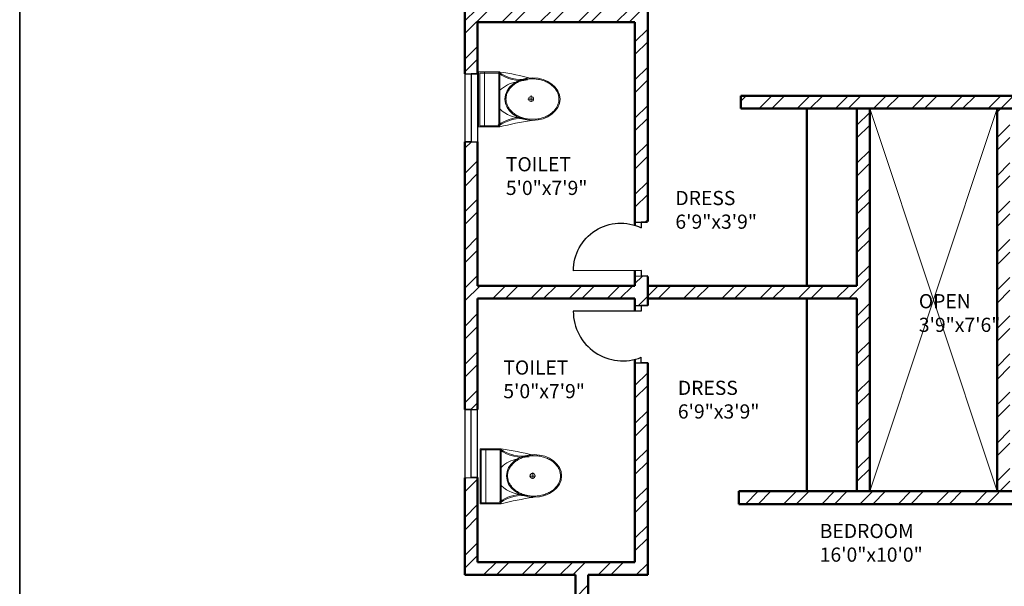
# Model space of a CAD drawing. Units: inches. Extents: x 963 to 2075, y 289 to 2657.
# Tile 16 of 98: x 963 to 1310, y 1917 to 2117. Entities that reach past the tile are written whole.
import ezdxf

# ---------------------------------------------------------------- set-up
doc = ezdxf.new("R2010")
doc.units = ezdxf.units.IN
for name, color, linetype, lineweight in [('A-ANNO-SYMB', 2, 'Continuous', 18), ('A-ANNO-TTLB', 7, 'Continuous', 35), ('A-AREA-IDEN', 7, 'Continuous', 18), ('A-DOOR', 4, 'Continuous', 25), ('A-FLOR-FIXT', 9, 'Continuous', 18), ('A-GLAZ', 3, 'Continuous', 25), ('A-WALL', 7, 'Continuous', 50), ('A-WALL-PATT', 8, 'Continuous', 13)]:
    doc.layers.add(name, color=color, linetype=linetype, lineweight=lineweight)
doc.styles.get("Standard").update_dxf_attribs({"font": 'arial.ttf'})

# ---------------------------------------------------------------- blocks, each defined once
blk = doc.blocks.new('A$C31115884')
for p, q in [((283.1, 497.7), (223.4, 497.7)), ((257.5, 466.4), (257.5, 523.2)), ((0, 200), (0, 0)), ((520, 200), (0, 200)), ((10, 190), (10, 10)), ((510, 190), (10, 190)), ((510, 10), (510, 190)), ((520, 0), (520, 200)), ((510, 54.5), (0, 54.5)), ((10, 10), (510, 10)), ((0, 0), (520, 0))]:
    blk.add_line(p, q)
blk.add_circle((255.6, 496.4), 23.6)
for centre, radius, start, end in [((2777.7, -204.6), 2807, 165.4549, 171.71327), ((3237, 905), 2807, 188.28673, 194.5451), ((-294.5, 403.3), 364.7, 324.20913, 9.34987), ((-294.5, 403.3), 374.7, 324.20913, 9.34987), ((139.5, 406.2), 293.5, 315.84364, 2.65635), ((805.8, 403.3), 374.7, 179.20365, 215.79087), ((805.8, 403.3), 364.7, 170.65013, 215.79087), ((383.6, 406.2), 293.5, 190.27735, 224.15636)]:
    blk.add_arc(centre, radius, start, end)
blk.add_ellipse((256.2, 509.9), major_axis=(0, -260.7), ratio=0.772727)
blk.add_open_spline([(256.2, 259.2), (263.1, 259.2), (270, 259.7), (287.8, 262.3), (298.7, 265.1), (319.9, 273.1), (330.2, 278.4), (350.1, 291.1), (359.7, 298.7), (377.7, 315.9), (386.2, 325.5), (401.7, 346.6), (408.8, 358.1), (421.3, 382.5), (426.8, 395.5), (435.9, 422.4), (439.5, 436.4), (444.8, 465.1), (446.5, 479.7), (447.9, 509.2), (447.6, 524), (445, 553.3), (442.7, 567.8), (436.3, 596), (432.1, 609.7), (421.9, 636), (416, 648.6), (402.5, 672.1), (395, 683), (378.6, 703), (369.8, 712.1), (351.1, 728), (341.3, 734.8), (320.9, 746.2), (310.4, 750.7), (288.9, 757.3), (278, 759.4), (256, 761), (245, 760.6), (223.1, 757.2), (212.3, 754.3), (191.1, 746.1), (180.8, 740.7), (160.9, 727.8), (151.4, 720.1), (133.5, 702.7), (125.1, 693), (109.6, 671.7), (102.6, 660.2), (90.2, 635.7), (84.9, 622.7), (76, 595.6), (72.4, 581.6), (67.2, 552.9), (65.6, 538.2), (64.4, 508.8), (64.8, 494), (67.5, 464.7), (69.9, 450.2), (76.6, 422), (80.8, 408.3), (91.1, 382.2), (97.2, 369.7), (110.8, 346.3), (118.4, 335.4), (134.8, 315.6), (143.7, 306.7), (162.4, 290.9), (172.3, 284.2), (192.8, 273), (203.3, 268.6), (224.8, 262.2), (235.8, 260.2), (249.9, 259.3), (253, 259.2), (256.2, 259.2)], degree=3, knots=[0, 0, 0, 0, 0.110105, 0.110105, 0.285049, 0.285049, 0.459994, 0.459994, 0.634938, 0.634938, 0.809882, 0.809882, 0.984827, 0.984827, 1.159771, 1.159771, 1.334715, 1.334715, 1.50966, 1.50966, 1.684604, 1.684604, 1.859549, 1.859549, 2.034493, 2.034493, 2.209437, 2.209437, 2.384382, 2.384382, 2.559326, 2.559326, 2.73427, 2.73427, 2.909215, 2.909215, 3.084159, 3.084159, 3.259103, 3.259103, 3.434048, 3.434048, 3.608992, 3.608992, 3.783936, 3.783936, 3.958881, 3.958881, 4.133825, 4.133825, 4.30877, 4.30877, 4.483714, 4.483714, 4.658658, 4.658658, 4.833603, 4.833603, 5.008547, 5.008547, 5.183491, 5.183491, 5.358436, 5.358436, 5.53338, 5.53338, 5.708324, 5.708324, 5.883269, 5.883269, 6.058213, 6.058213, 6.233158, 6.233158, 6.283185, 6.283185, 6.283185, 6.283185])
blk = doc.blocks.new('DOOR-4')
for p, q in [((16.99, 2.25), (16.99, 26.25)), ((0, 4.5), (0, 0)), ((18.99, 4.5), (18.99, 0)), ((0, 0), (0, 2.25)), ((0, 2.25), (2, 2.25)), ((18.99, 2.25), (16.99, 2.25)), ((18.99, 0), (18.99, 2.25))]:
    blk.add_line(p, q)
blk.add_arc((16.99, 9.57), 16.68, 90, 206.0308)

msp = doc.modelspace()

# ---------------------------------------------------------------- hatches: boundary and pattern name
at = {"layer": 'A-WALL-PATT'}
h = msp.add_hatch(dxfattribs=at)
h.set_pattern_fill('ANSI32', color=256)
h.paths.add_polyline_path([(1296.92, 2558.32), (1203.92, 2558.32), (1203.92, 2493.82), (1191.53, 2493.82), (1191.53, 2489.32), (1211.06, 2489.32), (1211.06, 2492.02), (1211.06, 2493.82), (1208.42, 2493.82), (1208.42, 2553.82), (1292.42, 2553.82), (1292.42, 2538.86), (1296.92, 2538.86)])
h.paths.add_polyline_path([(1442.42, 2558.32), (1349.42, 2558.32), (1349.42, 2538.94), (1353.92, 2538.94), (1353.92, 2553.82), (1437.92, 2553.82), (1437.92, 2493.82), (1434.54, 2493.82), (1434.54, 2489.32), (1448.31, 2489.32), (1448.31, 2491.57), (1448.31, 2493.82), (1442.42, 2493.82)])
h.paths.add_polyline_path([(1415.55, 2491.57), (1415.55, 2493.82), (1340.94, 2493.82), (1340.94, 2489.32), (1371.92, 2489.32), (1371.92, 2378.32), (1367.6, 2378.32), (1367.6, 2373.82), (1371.92, 2373.82), (1371.92, 2355.19), (1376.42, 2355.19), (1376.42, 2489.32), (1415.55, 2489.32)])
h.paths.add_polyline_path([(1304.94, 2491.57), (1304.94, 2493.82), (1296.92, 2493.82), (1296.92, 2514.86), (1292.42, 2514.86), (1292.42, 2493.82), (1232.81, 2493.82), (1232.81, 2489.32), (1256.42, 2489.32), (1256.42, 2327.32), (1253.71, 2327.32), (1253.71, 2322.82), (1328.42, 2322.82), (1328.42, 2331.15), (1323.92, 2331.15), (1323.92, 2327.32), (1260.92, 2327.32), (1260.92, 2373.82), (1323.92, 2373.82), (1323.92, 2357.81), (1328.42, 2357.81), (1328.42, 2373.82), (1346.01, 2373.82), (1346.01, 2376.07), (1346.01, 2378.32), (1260.92, 2378.32), (1260.92, 2489.32), (1304.94, 2489.32)])
h.paths.add_polyline_path([(1226.65, 2327.32), (1124.42, 2327.32), (1124.42, 2347.45), (1119.92, 2347.45), (1119.92, 2322.82), (1163.42, 2322.82), (1163.42, 2305.43), (1165.67, 2305.43), (1167.92, 2305.43), (1167.92, 2322.82), (1226.65, 2322.82), (1226.65, 2325.07)])
h.paths.add_polyline_path([(1095.92, 2489.32), (1124.42, 2489.32), (1131.53, 2489.32), (1131.53, 2491.57), (1131.53, 2493.82), (1119.92, 2493.82), (1091.42, 2493.82), (1091.42, 2417.32), (1095.92, 2417.32), (1119.92, 2417.32), (1119.92, 2407.45), (1124.42, 2407.45), (1124.42, 2421.82), (1095.92, 2421.82)])
h.paths.add_polyline_path([(1512.92, 2558.32), (1508.42, 2558.32), (1508.42, 2493.82), (1503.4, 2493.82), (1503.4, 2489.32), (1508.42, 2489.32), (1508.42, 2327.32), (1376.42, 2327.32), (1376.42, 2330.27), (1371.92, 2330.27), (1371.92, 2298.74), (1376.42, 2298.74), (1376.42, 2322.82), (1508.42, 2322.82), (1508.42, 2165.32), (1504.26, 2165.32), (1504.26, 2160.82), (1508.42, 2160.82), (1508.42, 2108.32), (1512.92, 2108.32), (1512.92, 2160.82), (1516.18, 2160.82), (1516.18, 2163.07), (1516.18, 2165.32), (1512.92, 2165.32), (1512.92, 2322.82), (1644.92, 2322.82), (1644.92, 2298.74), (1649.42, 2298.74), (1649.42, 2322.82), (1649.42, 2330.94), (1647.17, 2330.94), (1644.92, 2330.94), (1644.92, 2327.32), (1512.92, 2327.32), (1512.92, 2489.32), (1516.76, 2489.32), (1516.76, 2491.57), (1516.76, 2493.82), (1512.92, 2493.82)])
h.paths.add_polyline_path([(1671.92, 2558.32), (1578.92, 2558.32), (1578.92, 2493.82), (1573.53, 2493.82), (1573.53, 2489.32), (1586.54, 2489.32), (1586.54, 2491.57), (1586.54, 2493.82), (1583.42, 2493.82), (1583.42, 2553.82), (1667.42, 2553.82), (1667.42, 2541.11), (1671.92, 2541.11)])
h.paths.add_polyline_path([(1681.26, 2493.82), (1671.92, 2493.82), (1671.92, 2517.11), (1667.42, 2517.11), (1667.42, 2493.82), (1610.22, 2493.82), (1610.22, 2489.32), (1644.92, 2489.32), (1644.92, 2357.87), (1649.42, 2357.87), (1649.42, 2373.82), (1652.2, 2373.82), (1652.2, 2375.83), (1652.2, 2378.32), (1649.42, 2378.32), (1649.42, 2489.32), (1681.26, 2489.32), (1681.26, 2491.57)])
h.paths.add_polyline_path([(1821.92, 2558.32), (1728.92, 2558.32), (1728.92, 2541), (1733.42, 2541), (1733.42, 2553.82), (1817.42, 2553.82), (1817.42, 2493.82), (1813.51, 2493.82), (1813.51, 2489.32), (1830.08, 2489.32), (1830.08, 2491.57), (1830.08, 2493.82), (1821.92, 2493.82)])
h.paths.add_polyline_path([(1794.24, 2493.82), (1717.26, 2493.82), (1717.26, 2489.32), (1760.42, 2489.32), (1760.42, 2378.32), (1674.4, 2378.32), (1674.4, 2373.82), (1692.92, 2373.82), (1692.92, 2356.95), (1697.42, 2356.95), (1697.42, 2373.82), (1760.42, 2373.82), (1760.42, 2327.32), (1697.42, 2327.32), (1697.42, 2333.34), (1692.92, 2333.34), (1692.92, 2322.82), (1768.04, 2322.82), (1768.04, 2325.07), (1768.04, 2327.32), (1764.92, 2327.32), (1764.92, 2489.32), (1794.24, 2489.32)])
h.paths.add_polyline_path([(1733.42, 2517), (1728.92, 2517), (1728.92, 2493.82), (1733.42, 2493.82)], flags=17)
h.paths.add_polyline_path([(1929.92, 2493.82), (1890.08, 2493.82), (1890.08, 2489.32), (1896.92, 2489.32), (1925.42, 2489.32), (1925.42, 2421.82), (1896.92, 2421.82), (1896.92, 2408.32), (1901.42, 2408.32), (1901.42, 2417.32), (1925.42, 2417.32), (1929.92, 2417.32)])
h.paths.add_polyline_path([(1901.42, 2348.32), (1896.92, 2348.32), (1896.92, 2327.32), (1800.42, 2327.32), (1800.42, 2322.82), (1853.42, 2322.82), (1853.42, 2309.45), (1857.92, 2309.45), (1857.92, 2322.82), (1901.42, 2322.82)])
h.paths.add_polyline_path([(1857.92, 2249.45), (1853.42, 2249.45), (1853.42, 2214.82), (1686.31, 2214.82), (1686.31, 2210.32), (1853.42, 2210.32), (1853.42, 2202.13), (1857.92, 2202.13), (1857.92, 2210.32)])
h.paths.add_polyline_path([(1857.92, 2142.13), (1853.42, 2142.13), (1853.42, 2115.42), (1841.42, 2115.42), (1841.42, 2088.53), (1841.42, 2046.95), (1845.92, 2046.95), (1845.92, 2110.92), (1905.92, 2110.92), (1905.92, 2092.52), (1910.42, 2092.52), (1910.42, 2115.42), (1857.92, 2115.42)])
h.paths.add_polyline_path([(1532.44, 1482.34), (1573.46, 1482.34), (1573.46, 1501), (1532.44, 1501)], flags=9)
h.paths.add_polyline_path([(1438.66, 1486.3), (1479.68, 1486.3), (1479.68, 1504.96), (1438.66, 1504.96)], flags=9)
h.paths.add_polyline_path([(1411.22, 1365.31), (1659.14, 1365.31), (1659.14, 1402.4), (1411.22, 1402.4)], flags=9)
h.paths.add_polyline_path([(1185.67, 2296.3), (1248.16, 2296.3), (1248.16, 2314.95), (1185.67, 2314.95)], flags=9)
h.paths.add_polyline_path([(1177.31, 2187.35), (1216.15, 2187.35), (1216.15, 2206.01), (1177.31, 2206.01)], flags=9)
h.paths.add_polyline_path([(1295.1, 1602.08), (1328.26, 1602.08), (1328.26, 1620.74), (1295.1, 1620.74)], flags=9)
h.paths.add_polyline_path([(1525.13, 2005.99), (1558.39, 2005.99), (1558.39, 2024.65), (1525.13, 2024.65)], flags=9)
h.paths.add_polyline_path([(1459.61, 1977.13), (1472.19, 1977.13), (1472.19, 1987.43), (1459.61, 1987.43)], flags=9)
h.paths.add_polyline_path([(1467.81, 2053.68), (1480.02, 2053.68), (1480.02, 2063.98), (1467.81, 2063.98)], flags=9)
h.paths.add_polyline_path([(1555.18, 2119.02), (1584.56, 2119.02), (1584.56, 2137.68), (1555.18, 2137.68)], flags=25)
h.paths.add_polyline_path([(1405.39, 2115.29), (1444.48, 2115.29), (1444.48, 2133.95), (1405.39, 2133.95)], flags=25)
h.paths.add_polyline_path([(1698.48, 2004.26), (1727.69, 2004.26), (1727.69, 2022.92), (1698.48, 2022.92)], flags=9)
h.paths.add_polyline_path([(1612.16, 1972.86), (1629.02, 1972.86), (1629.02, 1983.16), (1612.16, 1983.16)], flags=9)
h.paths.add_polyline_path([(1608.29, 2060.04), (1625.15, 2060.04), (1625.15, 2070.34), (1608.29, 2070.34)], flags=9)
h.paths.add_polyline_path([(1527.95, 1684.4), (1566.79, 1684.4), (1566.79, 1703.06), (1527.95, 1703.06)], flags=9)
h.paths.add_polyline_path([(1422.79, 1683.59), (1461.63, 1683.59), (1461.63, 1702.25), (1422.79, 1702.25)], flags=9)
h.paths.add_polyline_path([(1531.26, 1732.46), (1574.01, 1732.46), (1574.01, 1751.12), (1531.26, 1751.12)], flags=9)
h.paths.add_polyline_path([(1402.87, 1732.85), (1439.8, 1732.85), (1439.8, 1751.5), (1402.87, 1751.5)], flags=9)
h.paths.add_polyline_path([(1243.12, 1923.13), (1281.96, 1923.13), (1281.96, 1941.79), (1243.12, 1941.79)], flags=9)
h.paths.add_polyline_path([(1181.75, 1792.27), (1244.24, 1792.27), (1244.24, 1810.93), (1181.75, 1810.93)], flags=9)
h.paths.add_polyline_path([(1265.82, 1670.3), (1316.07, 1670.3), (1316.07, 1688.96), (1265.82, 1688.96)], flags=9)
h.paths.add_polyline_path([(1140.26, 1676.05), (1179.1, 1676.05), (1179.1, 1694.71), (1140.26, 1694.71)], flags=9)
h.paths.add_polyline_path([(1107.49, 1490.89), (1143.37, 1490.89), (1143.37, 1509.55), (1107.49, 1509.55)], flags=9)
h.paths.add_polyline_path([(1217.58, 1483.9), (1246.74, 1483.9), (1246.74, 1502.56), (1217.58, 1502.56)], flags=9)
h.paths.add_polyline_path([(1389.21, 1486.92), (1418.37, 1486.92), (1418.37, 1505.58), (1389.21, 1505.58)], flags=9)
h.paths.add_polyline_path([(1672.21, 1602.08), (1705.37, 1602.08), (1705.37, 1620.74), (1672.21, 1620.74)], flags=9)
h.paths.add_polyline_path([(1752.08, 1522.64), (1781.24, 1522.64), (1781.24, 1541.3), (1752.08, 1541.3)], flags=9)
h.paths.add_polyline_path([(1848.27, 1491.26), (1884.16, 1491.26), (1884.16, 1509.92), (1848.27, 1509.92)], flags=9)
h.paths.add_polyline_path([(1822.47, 1685.62), (1861.31, 1685.62), (1861.31, 1704.28), (1822.47, 1704.28)], flags=9)
h.paths.add_polyline_path([(1713.19, 1672.23), (1763.44, 1672.23), (1763.44, 1690.89), (1713.19, 1690.89)], flags=9)
h.paths.add_polyline_path([(1736.62, 1790.58), (1799.11, 1790.58), (1799.11, 1809.24), (1736.62, 1809.24)], flags=9)
h.paths.add_polyline_path([(1691.49, 1916.36), (1730.33, 1916.36), (1730.33, 1935.01), (1691.49, 1935.01)], flags=9)
h.paths.add_polyline_path([(1764.87, 1973.92), (1794.31, 1973.92), (1794.31, 1992.58), (1764.87, 1992.58)], flags=9)
h.paths.add_polyline_path([(1767.85, 2034.02), (1797.29, 2034.02), (1797.29, 2052.67), (1767.85, 2052.67)], flags=9)
h.paths.add_polyline_path([(1851.59, 2060.33), (1880.75, 2060.33), (1880.75, 2078.99), (1851.59, 2078.99)], flags=25)
h.paths.add_polyline_path([(1688.49, 2086.87), (1727.33, 2086.87), (1727.33, 2105.53), (1688.49, 2105.53)], flags=9)
h.paths.add_polyline_path([(1537.74, 2293.58), (1580.49, 2293.58), (1580.49, 2312.24), (1537.74, 2312.24)], flags=25)
h.paths.add_polyline_path([(1425.59, 2296.11), (1468.34, 2296.11), (1468.34, 2314.77), (1425.59, 2314.77)], flags=25)
h.paths.add_polyline_path([(1278.52, 2004.18), (1307.72, 2004.18), (1307.72, 2022.84), (1278.52, 2022.84)], flags=9)
h.paths.add_polyline_path([(1193.28, 1973.63), (1222.72, 1973.63), (1222.72, 1992.29), (1193.28, 1992.29)], flags=9)
h.paths.add_polyline_path([(1192.41, 2040.58), (1221.84, 2040.58), (1221.84, 2059.23), (1192.41, 2059.23)], flags=9)
h.paths.add_polyline_path([(1130.6, 1951.39), (1159.76, 1951.39), (1159.76, 1970.05), (1130.6, 1970.05)], flags=9)
h.paths.add_polyline_path([(1132.83, 2052.49), (1161.98, 2052.49), (1161.98, 2071.15), (1132.83, 2071.15)], flags=9)
h.paths.add_polyline_path([(1265.13, 2334.62), (1315.38, 2334.62), (1315.38, 2353.28), (1265.13, 2353.28)], flags=25)
h.paths.add_polyline_path([(1136.74, 2330.79), (1175.58, 2330.79), (1175.58, 2349.44), (1136.74, 2349.44)], flags=9)
h.paths.add_polyline_path([(1287.42, 2417.2), (1320.58, 2417.2), (1320.58, 2435.86), (1287.42, 2435.86)], flags=25)
h.paths.add_polyline_path([(1430.99, 2329.16), (1469.83, 2329.16), (1469.83, 2347.82), (1430.99, 2347.82)], flags=25)
h.paths.add_polyline_path([(1525.42, 2329.21), (1564.26, 2329.21), (1564.26, 2347.87), (1525.42, 2347.87)], flags=25)
h.paths.add_polyline_path([(1684.52, 2382.8), (1717.68, 2382.8), (1717.68, 2401.46), (1684.52, 2401.46)], flags=25)
h.paths.add_polyline_path([(1704.81, 2340.29), (1755.05, 2340.29), (1755.05, 2358.95), (1704.81, 2358.95)], flags=25)
h.paths.add_polyline_path([(1694.11, 2287.76), (1756.6, 2287.76), (1756.6, 2306.41), (1694.11, 2306.41)], flags=9)
h.paths.add_polyline_path([(1815.78, 2329.86), (1854.62, 2329.86), (1854.62, 2348.52), (1815.78, 2348.52)], flags=9)
h.paths.add_polyline_path([(1842.87, 2514.26), (1878.76, 2514.26), (1878.76, 2532.91), (1842.87, 2532.91)], flags=9)
h.paths.add_polyline_path([(1769.51, 2531.45), (1798.67, 2531.45), (1798.67, 2550.1), (1769.51, 2550.1)], flags=25)
h.paths.add_polyline_path([(1594.77, 2518.47), (1623.93, 2518.47), (1623.93, 2537.13), (1594.77, 2537.13)], flags=25)
h.paths.add_polyline_path([(1520.72, 2516.18), (1556.61, 2516.18), (1556.61, 2534.84), (1520.72, 2534.84)], flags=25)
h.paths.add_polyline_path([(1464.46, 2516.69), (1500.34, 2516.69), (1500.34, 2535.35), (1464.46, 2535.35)], flags=25)
h.paths.add_polyline_path([(1365.7, 2528.97), (1394.85, 2528.97), (1394.85, 2547.63), (1365.7, 2547.63)], flags=25)
h.paths.add_polyline_path([(1222.84, 2516.23), (1252, 2516.23), (1252, 2534.89), (1222.84, 2534.89)], flags=25)
h.paths.add_polyline_path([(1104.55, 2509.6), (1140.43, 2509.6), (1140.43, 2528.26), (1104.55, 2528.26)], flags=9)
h = msp.add_hatch(dxfattribs=at)
h.set_pattern_fill('ANSI32', color=256)
h.paths.add_polyline_path([(1335.97, 2212.57), (1335.97, 2214.82), (1167.92, 2214.82), (1167.92, 2245.43), (1163.42, 2245.43), (1163.42, 2210.32), (1163.42, 2194.81), (1167.92, 2194.81), (1167.92, 2210.32), (1335.97, 2210.32)])
h.paths.add_polyline_path([(1532.44, 1482.34), (1573.46, 1482.34), (1573.46, 1501), (1532.44, 1501)], flags=9)
h.paths.add_polyline_path([(1438.66, 1486.3), (1479.68, 1486.3), (1479.68, 1504.96), (1438.66, 1504.96)], flags=9)
h.paths.add_polyline_path([(1411.22, 1365.31), (1659.14, 1365.31), (1659.14, 1402.4), (1411.22, 1402.4)], flags=9)
h.paths.add_polyline_path([(1185.67, 2296.3), (1248.16, 2296.3), (1248.16, 2314.95), (1185.67, 2314.95)], flags=9)
h.paths.add_polyline_path([(1177.31, 2187.35), (1216.15, 2187.35), (1216.15, 2206.01), (1177.31, 2206.01)], flags=9)
h.paths.add_polyline_path([(1295.1, 1602.08), (1328.26, 1602.08), (1328.26, 1620.74), (1295.1, 1620.74)], flags=9)
h.paths.add_polyline_path([(1525.13, 2005.99), (1558.39, 2005.99), (1558.39, 2024.65), (1525.13, 2024.65)], flags=9)
h.paths.add_polyline_path([(1459.61, 1977.13), (1472.19, 1977.13), (1472.19, 1987.43), (1459.61, 1987.43)], flags=9)
h.paths.add_polyline_path([(1467.81, 2053.68), (1480.02, 2053.68), (1480.02, 2063.98), (1467.81, 2063.98)], flags=9)
h.paths.add_polyline_path([(1555.18, 2119.02), (1584.56, 2119.02), (1584.56, 2137.68), (1555.18, 2137.68)], flags=9)
h.paths.add_polyline_path([(1405.39, 2115.29), (1444.48, 2115.29), (1444.48, 2133.95), (1405.39, 2133.95)], flags=9)
h.paths.add_polyline_path([(1698.48, 2004.26), (1727.69, 2004.26), (1727.69, 2022.92), (1698.48, 2022.92)], flags=9)
h.paths.add_polyline_path([(1612.16, 1972.86), (1629.02, 1972.86), (1629.02, 1983.16), (1612.16, 1983.16)], flags=9)
h.paths.add_polyline_path([(1608.29, 2060.04), (1625.15, 2060.04), (1625.15, 2070.34), (1608.29, 2070.34)], flags=9)
h.paths.add_polyline_path([(1527.95, 1684.4), (1566.79, 1684.4), (1566.79, 1703.06), (1527.95, 1703.06)], flags=9)
h.paths.add_polyline_path([(1422.79, 1683.59), (1461.63, 1683.59), (1461.63, 1702.25), (1422.79, 1702.25)], flags=9)
h.paths.add_polyline_path([(1531.26, 1732.46), (1574.01, 1732.46), (1574.01, 1751.12), (1531.26, 1751.12)], flags=9)
h.paths.add_polyline_path([(1402.87, 1732.85), (1439.8, 1732.85), (1439.8, 1751.5), (1402.87, 1751.5)], flags=9)
h.paths.add_polyline_path([(1243.12, 1923.13), (1281.96, 1923.13), (1281.96, 1941.79), (1243.12, 1941.79)], flags=9)
h.paths.add_polyline_path([(1181.75, 1792.27), (1244.24, 1792.27), (1244.24, 1810.93), (1181.75, 1810.93)], flags=9)
h.paths.add_polyline_path([(1265.82, 1670.3), (1316.07, 1670.3), (1316.07, 1688.96), (1265.82, 1688.96)], flags=9)
h.paths.add_polyline_path([(1140.26, 1676.05), (1179.1, 1676.05), (1179.1, 1694.71), (1140.26, 1694.71)], flags=9)
h.paths.add_polyline_path([(1107.49, 1490.89), (1143.37, 1490.89), (1143.37, 1509.55), (1107.49, 1509.55)], flags=9)
h.paths.add_polyline_path([(1217.58, 1483.9), (1246.74, 1483.9), (1246.74, 1502.56), (1217.58, 1502.56)], flags=9)
h.paths.add_polyline_path([(1389.21, 1486.92), (1418.37, 1486.92), (1418.37, 1505.58), (1389.21, 1505.58)], flags=9)
h.paths.add_polyline_path([(1672.21, 1602.08), (1705.37, 1602.08), (1705.37, 1620.74), (1672.21, 1620.74)], flags=9)
h.paths.add_polyline_path([(1752.08, 1522.64), (1781.24, 1522.64), (1781.24, 1541.3), (1752.08, 1541.3)], flags=9)
h.paths.add_polyline_path([(1848.27, 1491.26), (1884.16, 1491.26), (1884.16, 1509.92), (1848.27, 1509.92)], flags=9)
h.paths.add_polyline_path([(1822.47, 1685.62), (1861.31, 1685.62), (1861.31, 1704.28), (1822.47, 1704.28)], flags=9)
h.paths.add_polyline_path([(1713.19, 1672.23), (1763.44, 1672.23), (1763.44, 1690.89), (1713.19, 1690.89)], flags=9)
h.paths.add_polyline_path([(1736.62, 1790.58), (1799.11, 1790.58), (1799.11, 1809.24), (1736.62, 1809.24)], flags=9)
h.paths.add_polyline_path([(1691.49, 1916.36), (1730.33, 1916.36), (1730.33, 1935.01), (1691.49, 1935.01)], flags=9)
h.paths.add_polyline_path([(1764.87, 1973.92), (1794.31, 1973.92), (1794.31, 1992.58), (1764.87, 1992.58)], flags=9)
h.paths.add_polyline_path([(1767.85, 2034.02), (1797.29, 2034.02), (1797.29, 2052.67), (1767.85, 2052.67)], flags=9)
h.paths.add_polyline_path([(1851.59, 2060.33), (1880.75, 2060.33), (1880.75, 2078.99), (1851.59, 2078.99)], flags=9)
h.paths.add_polyline_path([(1688.49, 2086.87), (1727.33, 2086.87), (1727.33, 2105.53), (1688.49, 2105.53)], flags=9)
h.paths.add_polyline_path([(1537.74, 2293.58), (1580.49, 2293.58), (1580.49, 2312.24), (1537.74, 2312.24)], flags=9)
h.paths.add_polyline_path([(1425.59, 2296.11), (1468.34, 2296.11), (1468.34, 2314.77), (1425.59, 2314.77)], flags=9)
h.paths.add_polyline_path([(1278.52, 2004.18), (1307.72, 2004.18), (1307.72, 2022.84), (1278.52, 2022.84)], flags=9)
h.paths.add_polyline_path([(1193.28, 1973.63), (1222.72, 1973.63), (1222.72, 1992.29), (1193.28, 1992.29)], flags=9)
h.paths.add_polyline_path([(1192.41, 2040.58), (1221.84, 2040.58), (1221.84, 2059.23), (1192.41, 2059.23)], flags=9)
h.paths.add_polyline_path([(1130.6, 1951.39), (1159.76, 1951.39), (1159.76, 1970.05), (1130.6, 1970.05)], flags=9)
h.paths.add_polyline_path([(1132.83, 2052.49), (1161.98, 2052.49), (1161.98, 2071.15), (1132.83, 2071.15)], flags=9)
h.paths.add_polyline_path([(1265.13, 2334.62), (1315.38, 2334.62), (1315.38, 2353.28), (1265.13, 2353.28)], flags=9)
h.paths.add_polyline_path([(1136.74, 2330.79), (1175.58, 2330.79), (1175.58, 2349.44), (1136.74, 2349.44)], flags=9)
h.paths.add_polyline_path([(1287.42, 2417.2), (1320.58, 2417.2), (1320.58, 2435.86), (1287.42, 2435.86)], flags=9)
h.paths.add_polyline_path([(1430.99, 2329.16), (1469.83, 2329.16), (1469.83, 2347.82), (1430.99, 2347.82)], flags=9)
h.paths.add_polyline_path([(1525.42, 2329.21), (1564.26, 2329.21), (1564.26, 2347.87), (1525.42, 2347.87)], flags=9)
h.paths.add_polyline_path([(1684.52, 2382.8), (1717.68, 2382.8), (1717.68, 2401.46), (1684.52, 2401.46)], flags=9)
h.paths.add_polyline_path([(1704.81, 2340.29), (1755.05, 2340.29), (1755.05, 2358.95), (1704.81, 2358.95)], flags=9)
h.paths.add_polyline_path([(1694.11, 2287.76), (1756.6, 2287.76), (1756.6, 2306.41), (1694.11, 2306.41)], flags=9)
h.paths.add_polyline_path([(1815.78, 2329.86), (1854.62, 2329.86), (1854.62, 2348.52), (1815.78, 2348.52)], flags=9)
h.paths.add_polyline_path([(1842.87, 2514.26), (1878.76, 2514.26), (1878.76, 2532.91), (1842.87, 2532.91)], flags=9)
h.paths.add_polyline_path([(1769.51, 2531.45), (1798.67, 2531.45), (1798.67, 2550.1), (1769.51, 2550.1)], flags=9)
h.paths.add_polyline_path([(1594.77, 2518.47), (1623.93, 2518.47), (1623.93, 2537.13), (1594.77, 2537.13)], flags=9)
h.paths.add_polyline_path([(1520.72, 2516.18), (1556.61, 2516.18), (1556.61, 2534.84), (1520.72, 2534.84)], flags=9)
h.paths.add_polyline_path([(1464.46, 2516.69), (1500.34, 2516.69), (1500.34, 2535.35), (1464.46, 2535.35)], flags=9)
h.paths.add_polyline_path([(1365.7, 2528.97), (1394.85, 2528.97), (1394.85, 2547.63), (1365.7, 2547.63)], flags=9)
h.paths.add_polyline_path([(1222.84, 2516.23), (1252, 2516.23), (1252, 2534.89), (1222.84, 2534.89)], flags=9)
h.paths.add_polyline_path([(1104.55, 2509.6), (1140.43, 2509.6), (1140.43, 2528.26), (1104.55, 2528.26)], flags=9)
h = msp.add_hatch(dxfattribs=at)
h.set_pattern_fill('ANSI32', color=256)
h.paths.add_polyline_path([(1473.61, 2163.07), (1473.61, 2165.32), (1376.42, 2165.32), (1376.42, 2227.98), (1371.92, 2227.98), (1371.92, 2214.82), (1368.41, 2214.82), (1368.41, 2210.32), (1371.92, 2210.32), (1371.92, 2160.82), (1395.92, 2160.82), (1395.92, 2090.32), (1217.34, 2090.32), (1217.34, 2085.82), (1395.92, 2085.82), (1458.92, 2085.82), (1458.92, 2108.32), (1454.42, 2108.32), (1454.42, 2090.32), (1400.42, 2090.32), (1400.42, 2160.82), (1473.61, 2160.82)])
h.paths.add_polyline_path([(1649.42, 2210.32), (1653.23, 2210.32), (1653.23, 2214.82), (1649.42, 2214.82), (1649.42, 2227.98), (1644.92, 2227.98), (1644.92, 2165.32), (1550.1, 2165.32), (1550.1, 2160.82), (1620.92, 2160.82), (1620.92, 2112.82), (1555.45, 2112.82), (1555.45, 2108.32), (1584.33, 2108.32), (1584.33, 2084.92), (1588.83, 2084.92), (1588.83, 2108.32), (1625.42, 2108.32), (1667.95, 2108.32), (1667.95, 2022.67), (1588.83, 2022.67), (1588.83, 2047.41), (1584.33, 2047.41), (1584.33, 1996), (1588.83, 1996), (1588.83, 2018.32), (1667.95, 2018.17), (1667.95, 1928.32), (1625.42, 1928.32), (1625.42, 1923.82), (1672.45, 1923.82), (1672.45, 1928.32), (1672.45, 1946.66), (1785.45, 1946.66), (1785.45, 1951.16), (1743.03, 1951.16), (1743.03, 2017.92), (1841.42, 2017.92), (1841.42, 2014.77), (1845.92, 2014.77), (1845.92, 2017.92), (1905.92, 2017.92), (1905.92, 1987.51), (1910.42, 1987.51), (1910.42, 2022.42), (1910.42, 2068.52), (1905.92, 2068.52), (1905.92, 2022.42), (1845.92, 2022.42), (1845.92, 2025.85), (1843.67, 2025.85), (1841.42, 2025.85), (1841.42, 2022.42), (1743.03, 2022.42), (1743.03, 2084.03), (1768.45, 2084.03), (1785.45, 2084.03), (1785.45, 2088.53), (1672.45, 2088.53), (1672.45, 2112.82), (1667.95, 2112.82), (1625.42, 2112.82), (1625.42, 2160.82), (1649.42, 2160.82)])
h.paths.add_polyline_path([(1672.45, 2084.03), (1738.53, 2084.03), (1738.53, 1951.16), (1672.45, 1951.16)], flags=16)
h.paths.add_polyline_path([(1672.45, 2084.03), (1738.53, 2084.03), (1705.49, 2017.6)], flags=0)
h.paths.add_polyline_path([(1262.77, 2085.82), (1258.27, 2085.82), (1258.27, 2023.28), (1184.42, 2023.28), (1184.42, 2018.78), (1258.27, 2018.78), (1258.27, 1950.82), (1262.77, 1950.82)])
h.paths.add_polyline_path([(1312.27, 2085.82), (1307.77, 2085.82), (1307.77, 1950.82), (1312.27, 1950.82)])
h.paths.add_polyline_path([(1458.92, 1950.82), (1395.92, 1950.82), (1216.57, 1950.82), (1216.57, 1946.32), (1346.42, 1946.32), (1395.92, 1946.32), (1395.92, 1875.82), (1371.92, 1875.82), (1371.92, 1826.32), (1368.93, 1826.32), (1368.93, 1821.82), (1371.92, 1821.82), (1371.92, 1813.62), (1376.42, 1813.62), (1376.42, 1871.32), (1474.5, 1871.32), (1474.5, 1873.57), (1474.5, 1875.82), (1400.42, 1875.82), (1400.42, 1946.32), (1454.42, 1946.32), (1454.42, 1928.32), (1458.92, 1928.32)])
h.paths.add_polyline_path([(1184.42, 2120.78), (1167.92, 2120.78), (1167.92, 2134.81), (1165.67, 2134.81), (1163.42, 2134.81), (1163.42, 2120.78), (1119.92, 2120.78), (1119.92, 2098.1), (1124.42, 2098.1), (1124.42, 2116.28), (1167.92, 2116.28), (1179.92, 2116.28), (1179.92, 2045.92), (1184.42, 2045.92), (1184.42, 2090.32), (1184.42, 2116.28)])
h.paths.add_polyline_path([(1124.42, 2018.78), (1179.92, 2018.78), (1179.92, 2016.29), (1184.42, 2016.29), (1184.42, 2023.28), (1184.42, 2026.59), (1182.17, 2026.59), (1179.92, 2026.59), (1179.92, 2023.28), (1124.42, 2023.28), (1124.42, 2074.1), (1119.92, 2074.1), (1119.92, 2018.78), (1119.92, 1979.63), (1124.42, 1979.63)])
h.paths.add_polyline_path([(1184.42, 1925.78), (1184.42, 1946.32), (1184.42, 1996.07), (1182.17, 1996.07), (1179.92, 1996.07), (1179.92, 1925.78), (1124.42, 1925.78), (1124.42, 1955.63), (1119.92, 1955.5), (1119.92, 1921.28), (1158.92, 1921.28), (1158.92, 1909.98), (1163.42, 1909.98), (1163.42, 1921.28), (1184.42, 1921.28)])
h.paths.add_polyline_path([(1341.45, 1826.32), (1163.42, 1826.32), (1163.42, 1849.98), (1158.92, 1849.98), (1158.92, 1821.82), (1158.92, 1804.03), (1163.42, 1804.03), (1163.42, 1821.82), (1341.45, 1821.82)])
h.paths.add_polyline_path([(1222.98, 1713.82), (1163.42, 1713.82), (1163.42, 1744.03), (1161.17, 1744.03), (1158.92, 1744.03), (1158.92, 1713.82), (1119.92, 1713.82), (1119.92, 1694.65), (1124.42, 1694.65), (1124.42, 1709.32), (1158.92, 1709.32), (1222.98, 1709.32)])
h.paths.add_polyline_path([(1328.42, 1713.82), (1252.04, 1713.82), (1252.04, 1711.57), (1252.04, 1709.32), (1256.42, 1709.32), (1256.42, 1547.32), (1232.94, 1547.32), (1232.94, 1545.07), (1232.94, 1542.82), (1292.42, 1542.82), (1292.42, 1527.63), (1296.92, 1527.63), (1296.92, 1542.82), (1299.46, 1542.82), (1299.46, 1547.32), (1260.92, 1547.32), (1260.92, 1658.32), (1343.66, 1658.32), (1343.66, 1660.57), (1343.66, 1662.82), (1328.42, 1662.82), (1328.42, 1676.59), (1327.4, 1676.59), (1323.92, 1676.59), (1323.92, 1662.82), (1260.92, 1662.82), (1260.92, 1709.32), (1323.92, 1709.32), (1323.92, 1699.85), (1328.42, 1699.85)])
h.paths.add_polyline_path([(1649.42, 1875.82), (1625.42, 1875.82), (1625.42, 1928.32), (1620.92, 1928.32), (1588.83, 1928.32), (1588.83, 1950.59), (1584.33, 1950.59), (1584.33, 1928.32), (1555.45, 1928.32), (1555.45, 1923.82), (1620.92, 1923.82), (1620.92, 1875.82), (1548.95, 1875.82), (1548.95, 1873.57), (1548.95, 1871.32), (1644.92, 1871.32), (1644.92, 1813.62), (1649.42, 1813.62), (1649.42, 1821.82), (1652.04, 1821.82), (1652.04, 1824.07), (1652.04, 1826.32), (1649.42, 1826.32)])
h.paths.add_polyline_path([(1512.92, 1871.32), (1516.48, 1871.32), (1516.48, 1875.82), (1512.92, 1875.82), (1512.92, 1923.82), (1512.92, 1928.32), (1512.92, 1930.83), (1508.42, 1930.83), (1508.42, 1875.82), (1504.41, 1875.82), (1504.41, 1871.32), (1508.42, 1871.32), (1508.42, 1713.82), (1376.42, 1713.82), (1376.42, 1743.32), (1371.92, 1743.32), (1371.92, 1709.32), (1371.92, 1706.01), (1376.42, 1706.01), (1376.42, 1709.32), (1508.42, 1709.32), (1508.42, 1547.32), (1501.87, 1547.32), (1501.87, 1542.82), (1508.42, 1542.82), (1508.42, 1482.82), (1508.42, 1436.32), (1512.92, 1436.32), (1512.92, 1542.82), (1519.32, 1542.82), (1519.32, 1545.07), (1519.32, 1547.32), (1512.92, 1547.32), (1512.92, 1709.32), (1644.92, 1709.32), (1644.92, 1707.55), (1649.42, 1707.55), (1649.42, 1709.32), (1649.42, 1743.32), (1644.92, 1743.32), (1644.92, 1713.82), (1512.92, 1713.82)])
h.paths.add_polyline_path([(1129.88, 1545.07), (1129.88, 1547.32), (1124.42, 1547.32), (1095.92, 1547.32), (1095.92, 1614.82), (1124.42, 1614.82), (1124.42, 1619.32), (1095.92, 1619.32), (1091.42, 1619.32), (1091.42, 1542.82), (1095.92, 1542.82), (1119.92, 1542.82), (1129.88, 1542.82)])
h.paths.add_polyline_path([(1208.42, 1542.82), (1211.74, 1542.82), (1211.74, 1547.32), (1198.85, 1547.32), (1198.85, 1542.82), (1203.92, 1542.82), (1203.92, 1478.32), (1208.42, 1478.32), (1296.92, 1478.32), (1296.92, 1503.63), (1292.42, 1503.63), (1292.42, 1482.82), (1208.42, 1482.82)])
h.paths.add_polyline_path([(1430.42, 1542.82), (1435.7, 1542.82), (1435.7, 1545.07), (1435.7, 1547.32), (1422.66, 1547.32), (1422.66, 1545.07), (1422.66, 1542.82), (1425.92, 1542.82), (1425.92, 1482.86), (1341.92, 1482.86), (1341.92, 1502.73), (1337.42, 1502.73), (1337.42, 1478.36), (1425.92, 1478.36), (1425.92, 1440.82), (1425.92, 1436.32), (1430.42, 1436.32)])
h.paths.add_polyline_path([(1698.48, 2004.26), (1727.69, 2004.26), (1727.69, 2022.92), (1698.48, 2022.92)], flags=8)

# ---------------------------------------------------------------- linework, layer by layer
at = {"layer": 'A-ANNO-SYMB'}
for p, q in [((1307.77, 2085.82), (1262.77, 1950.82)), ((1307.77, 1950.82), (1262.77, 2085.82))]:
    msp.add_line(p, q, dxfattribs=at)
at = {"layer": 'A-ANNO-TTLB'}
msp.add_lwpolyline([(962.81, 2657.49), (2074.6, 2657.49), (2074.6, 1303.08), (962.81, 1303.08)], close=True, dxfattribs=at)
at = {"layer": 'A-DOOR'}
for p, q in [((1179.92, 2016.29), (1184.42, 2016.29)), ((1184.42, 2016.29), (1182.17, 2016.29)), ((1182.17, 2016.29), (1182.17, 2014.29)), ((1182.17, 2014.29), (1158.17, 2014.29)), ((1182.17, 1996.07), (1182.17, 1998.07)), ((1179.92, 1996.07), (1184.42, 1996.07)), ((1184.42, 1996.07), (1182.17, 1996.07))]:
    msp.add_line(p, q, dxfattribs=at)
msp.add_arc((1175.65, 2014.29), 17.48, 180, 291.8922, dxfattribs=at)
at = {"layer": 'A-GLAZ'}
for p, q in [((1119.92, 2098.1), (1124.42, 2098.1)), ((1119.92, 2098.1), (1119.92, 2074.1)), ((1124.42, 2098.1), (1122.17, 2098.1)), ((1122.17, 2098.1), (1122.17, 2074.1)), ((1124.42, 2098.1), (1124.42, 2074.1)), ((1122.17, 2074.1), (1119.92, 2074.1)), ((1119.92, 2074.1), (1124.42, 2074.1)), ((1122.17, 1979.63), (1119.92, 1979.63)), ((1119.92, 1979.63), (1124.42, 1979.63)), ((1119.92, 1979.63), (1119.92, 1955.5)), ((1122.17, 1955.63), (1122.17, 1979.63)), ((1124.42, 1955.63), (1124.42, 1979.63)), ((1119.92, 1955.5), (1124.42, 1955.63)), ((1124.42, 1955.63), (1122.17, 1955.63))]:
    msp.add_line(p, q, dxfattribs=at)
at = {"layer": 'A-WALL'}
for p, q in [((1119.92, 2120.78), (1119.92, 2098.1)), ((1184.42, 2116.28), (1184.42, 2120.78)), ((1124.42, 2116.28), (1124.42, 2098.1)), ((1124.42, 2116.28), (1167.92, 2116.28)), ((1124.42, 2098.1), (1124.42, 2116.28)), ((1167.92, 2116.28), (1179.92, 2116.28)), ((1179.92, 2116.28), (1179.92, 2044.77)), ((1184.42, 2090.32), (1184.42, 2116.28)), ((1184.42, 2045.92), (1184.42, 2090.32)), ((1395.92, 2090.32), (1217.34, 2090.32)), ((1217.34, 2090.32), (1217.34, 2090.32)), ((1217.34, 2090.32), (1217.34, 2085.82)), ((1217.34, 2085.82), (1395.92, 2085.82)), ((1275.17, 2085.82), (1230.17, 2085.82)), ((1240.54, 2085.82), (1240.54, 2023.28)), ((1258.27, 2023.28), (1258.27, 2085.82)), ((1262.77, 2085.82), (1262.77, 1950.82)), ((1307.77, 1950.82), (1307.77, 2085.82)), ((1119.92, 2074.1), (1119.92, 2018.78)), ((1124.42, 2023.28), (1124.42, 2074.1)), ((1124.42, 2074.1), (1124.42, 2023.28)), ((1179.92, 2028.59), (1179.92, 2023.28)), ((1184.42, 2023.28), (1184.42, 2026.59)), ((1179.92, 2023.28), (1124.42, 2023.28)), ((1258.27, 2023.28), (1184.42, 2023.28)), ((1184.42, 2016.29), (1184.42, 2023.28)), ((1119.92, 2018.78), (1119.92, 1979.63)), ((1124.42, 2018.78), (1179.92, 2018.78)), ((1124.42, 2018.78), (1124.42, 1979.63)), ((1179.92, 2014.29), (1179.92, 2018.78)), ((1184.42, 2018.78), (1258.27, 2018.78)), ((1240.54, 2018.78), (1240.54, 1950.82)), ((1258.27, 1950.82), (1258.27, 2018.78)), ((1179.92, 1925.78), (1179.92, 1997.34)), ((1184.42, 1946.32), (1184.42, 1996.07)), ((1119.92, 1955.5), (1119.92, 1921.28)), ((1124.42, 1955.63), (1124.42, 1925.78)), ((1216.57, 1950.82), (1395.92, 1950.82)), ((1216.57, 1950.82), (1216.57, 1946.32)), ((1230.17, 1950.82), (1225.67, 1950.82)), ((1279.67, 1950.82), (1275.17, 1950.82)), ((1184.42, 1925.78), (1184.42, 1946.32)), ((1216.57, 1946.32), (1346.42, 1946.32)), ((1124.42, 1925.78), (1179.92, 1925.78)), ((1184.42, 1921.28), (1184.42, 1925.78)), ((1119.92, 1921.28), (1158.92, 1921.28)), ((1158.92, 1909.98), (1158.92, 1921.28)), ((1163.42, 1921.28), (1163.42, 1909.98)), ((1163.42, 1921.28), (1184.42, 1921.28)), ((1184.42, 1921.28), (1179.92, 1921.28))]:
    msp.add_line(p, q, dxfattribs=at)

# ---------------------------------------------------------------- block references
at = {"layer": 'A-DOOR', "extrusion": (0, 0, -1), "zscale": -1, "rotation": 269.6581722131579}
msp.add_blockref('DOOR-4', (-1184.37, 2045.75), dxfattribs=at)
at = {"layer": 'A-FLOR-FIXT', "xscale": 0.0372717239612423, "yscale": 0.0372717239612423, "zscale": 0.0372717239612423, "rotation": 270}
for p in [(1124.76, 2098.71), (1125.31, 1965.78)]:
    msp.add_blockref('A$C31115884', p, dxfattribs=at)

# ---------------------------------------------------------------- texts
at = {"layer": 'A-AREA-IDEN', "char_height": 5, "attachment_point": 1}
for s, width, insert in [('TOILET\\P5\'0"x7\'9"', 96.8421, (1134.37, 2068.67)), ('DRESS\\P6\'9"x3\'9"', 101.0019, (1194.2, 2056.75)), ('OPEN\\P3\'9"x7\'6"', 62.5172, (1280.11, 2020.36)), ('TOILET\\P5\'0"x7\'9"', 79.5847, (1133.48, 1996.96)), ('DRESS\\P6\'9"x3\'9"', 100.6018, (1195.07, 1989.8)), ('BEDROOM\\P16\'0"x10\'0"', 133.4037, (1245.13, 1939.3))]:
    msp.add_mtext_dynamic_manual_height_columns(s, width=width, gutter_width=12.5, heights=[0], dxfattribs=dict(at, insert=insert))

doc.saveas('drawing.dxf')
